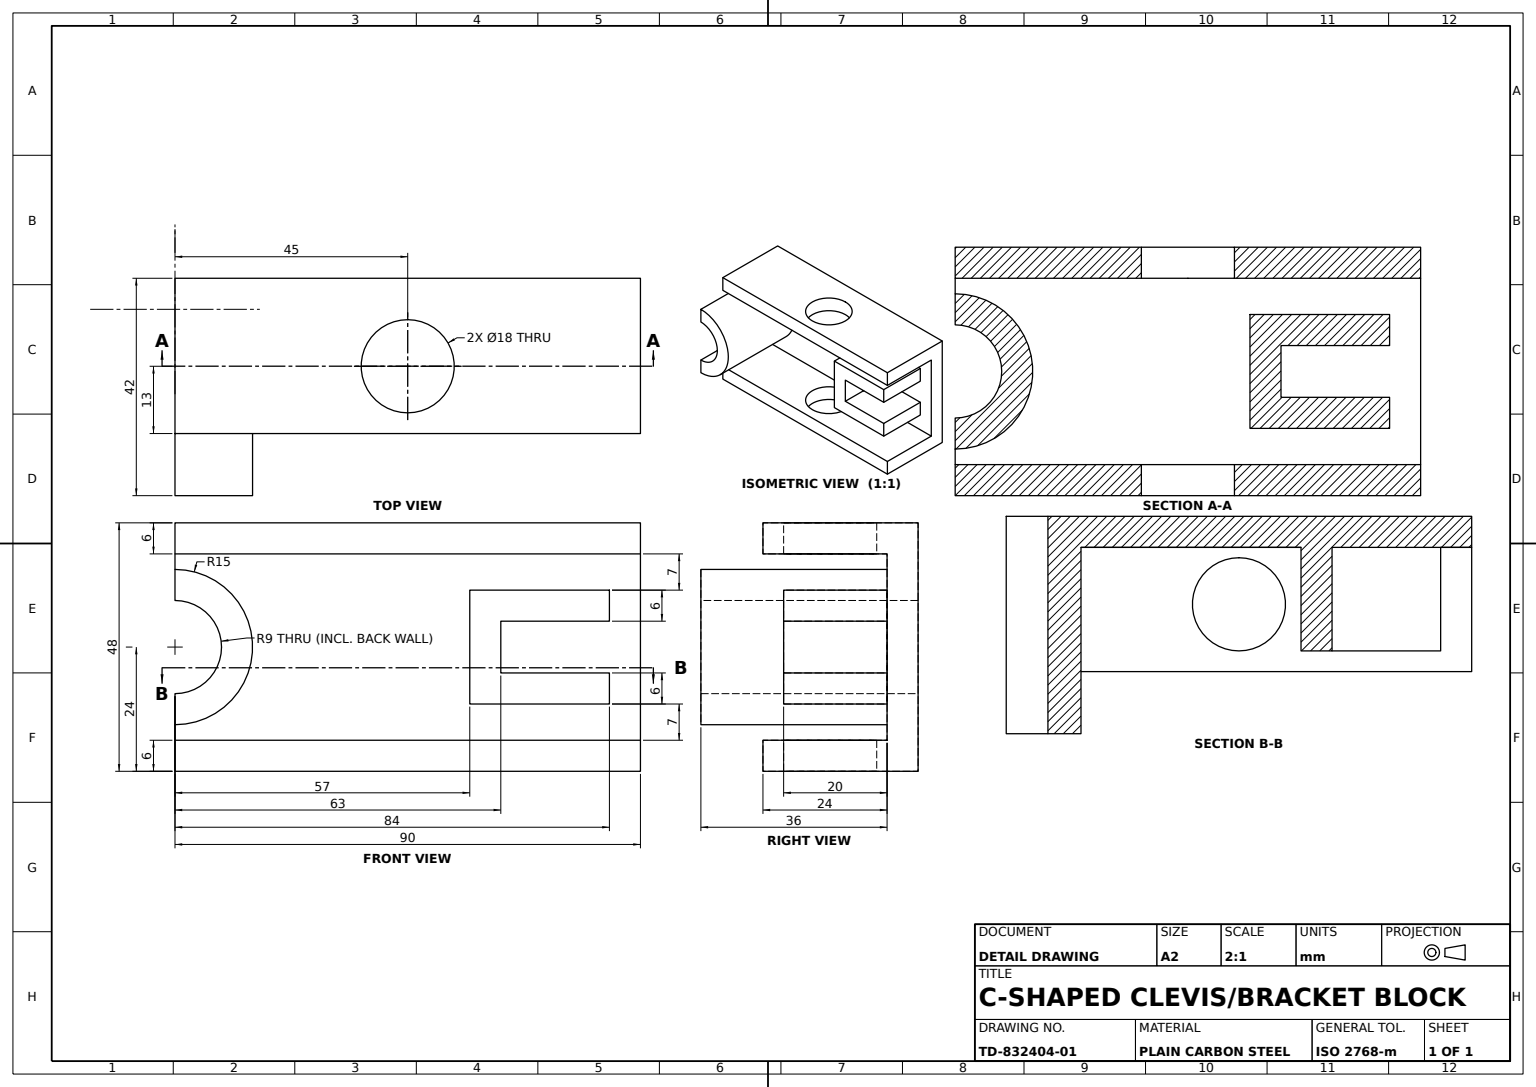
from build123d import *

# Parameters (mm, degrees)
BASE_BLOCK_SKETCH_W           = 90
BASE_BLOCK_SKETCH_H           = 48
BASE_BLOCK_DEPTH              = 30
CHANNEL_SLOT_SKETCH_W         = 78
CHANNEL_SLOT_SKETCH_H         = 36
CHANNEL_SLOT_DEPTH            = 24
CHANNEL_RELIEF_CUT_1_SKETCH_W = 6
CHANNEL_RELIEF_CUT_1_SKETCH_H = 36
CHANNEL_RELIEF_CUT_1_DEPTH    = 24
CHANNEL_RELIEF_CUT_2_SKETCH_W = 6
CHANNEL_RELIEF_CUT_2_SKETCH_H = 36
CHANNEL_RELIEF_CUT_2_DEPTH    = 24
HALF_CYLINDER_BOSS_DEPTH      = 36
BOSS_BORE_18_DEPTH            = 42
UPPER_PLATE_HOLE_SKETCH_R     = 9
UPPER_PLATE_HOLE_18_DEPTH     = 6
LOWER_START                   = -6
LOWER_PLATE_HOLE_SKETCH_R     = 9
LOWER_PLATE_HOLE_18_DEPTH     = 6
C_CLIP_BOSS_DEPTH             = 20


with BuildPart() as part:
    # Base Block Sketch → Base Block (new body)
    with BuildSketch(Plane.XY):
        with Locations((45, 24)):
            Rectangle(BASE_BLOCK_SKETCH_W, BASE_BLOCK_SKETCH_H)
    extrude(amount=BASE_BLOCK_DEPTH)

    # Channel Slot Sketch → Channel Slot (cut)
    with BuildSketch(Plane.XY.offset(30)):
        with Locations((45, 24)):
            Rectangle(CHANNEL_SLOT_SKETCH_W, CHANNEL_SLOT_SKETCH_H)
    extrude(amount=-CHANNEL_SLOT_DEPTH, mode=Mode.SUBTRACT)

    # Channel Relief Cut 1 Sketch → Channel Relief Cut 1 (cut)
    with BuildSketch(Plane.XY.offset(30)):
        with Locations((3, 24)):
            Rectangle(CHANNEL_RELIEF_CUT_1_SKETCH_W, CHANNEL_RELIEF_CUT_1_SKETCH_H)
    extrude(amount=-CHANNEL_RELIEF_CUT_1_DEPTH, mode=Mode.SUBTRACT)

    # Channel Relief Cut 2 Sketch → Channel Relief Cut 2 (cut)
    with BuildSketch(Plane.XY.offset(30)):
        with Locations((87, 24)):
            Rectangle(CHANNEL_RELIEF_CUT_2_SKETCH_W, CHANNEL_RELIEF_CUT_2_SKETCH_H)
    extrude(amount=-CHANNEL_RELIEF_CUT_2_DEPTH, mode=Mode.SUBTRACT)

    # Half Cylinder Boss Sketch → Half Cylinder Boss (add)
    with BuildSketch(Plane.XY.offset(6)):
        with BuildLine():
            Line((0, 39), (0, 9))
            ThreePointArc((0, 9), (15, 24), (0, 39))
        make_face()
    extrude(amount=HALF_CYLINDER_BOSS_DEPTH)

    # Boss Bore Sketch → Boss Bore Ø18 (cut)
    with BuildSketch(Plane.XY.offset(42)):
        with BuildLine():
            Line((0, 33), (0, 15))
            ThreePointArc((0, 15), (9, 24), (0, 33))
        make_face()
    extrude(amount=-BOSS_BORE_18_DEPTH, mode=Mode.SUBTRACT)

    # Upper Plate Hole Sketch → Upper Plate Hole Ø18 (cut)
    with BuildSketch(Plane.XZ):
        with Locations(Location((45, 17, 0), (0, 0, 270))):
            Circle(UPPER_PLATE_HOLE_SKETCH_R)
    extrude(amount=-UPPER_PLATE_HOLE_18_DEPTH, mode=Mode.SUBTRACT)

    # Lower Plate Hole Sketch → Lower Plate Hole Ø18 (cut)
    with BuildSketch(Plane(origin=(0, 48, 0), x_dir=(1, 0, 0), z_dir=(0, 1, 0)).offset(LOWER_START)):
        with Locations(Location((45, -17, 0), (0, 0, 90))):
            Circle(LOWER_PLATE_HOLE_SKETCH_R)
    extrude(amount=LOWER_PLATE_HOLE_18_DEPTH, mode=Mode.SUBTRACT)

    # C Clip Boss Sketch → C Clip Boss (add)
    with BuildSketch(Plane.XY.offset(6)):
        Polygon((84, 35), (84, 29), (63, 29), (63, 19), (84, 19), (84, 13), (57, 13), (57, 35), align=None)
    extrude(amount=C_CLIP_BOSS_DEPTH)


solid = part.part
